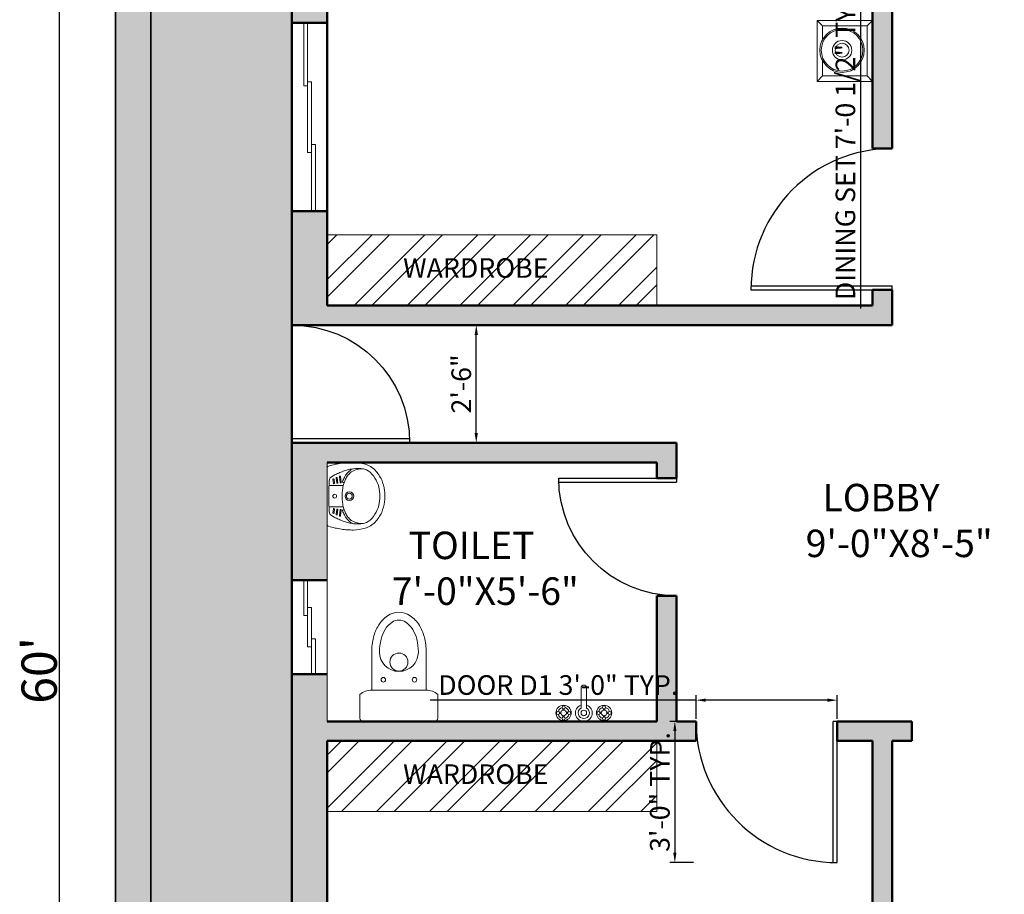
# Model space of a CAD drawing. Units: inches. Extents: x 1734 to 4011, y 1071 to 1891.
# Tile 16 of 27: x 3092 to 3343, y 1415 to 1638. Entities that reach past the tile are written whole.
import ezdxf

# ---------------------------------------------------------------- set-up
doc = ezdxf.new("R2010")
doc.units = ezdxf.units.IN
for name, color, linetype, lineweight in [('0.15', 34, 'Continuous', 15), ('A-ANNO-DIMS', 2, 'Continuous', 18), ('A-AREA-IDEN', 3, 'Continuous', 18), ('A-DOOR', 3, 'Continuous', 25), ('A-FLOR-FIXT', 9, 'Continuous', 18), ('A-FLOR-PATT', 252, 'Continuous', 13), ('A-FURN', 8, 'Continuous', 18), ('A-FURN-PATT', 252, 'Continuous', 13), ('A-GLAZ', 4, 'Continuous', 18), ('A-WALL', 7, 'Continuous', 50), ('A-WALL-PATT', 8, 'Continuous', 13), ('C-PROP', 1, 'Continuous', 35)]:
    doc.layers.add(name, color=color, linetype=linetype, lineweight=lineweight)
doc.styles.get("Standard").update_dxf_attribs({"font": 'arial.ttf'})
doc.dimstyles.new('ISO-25', dxfattribs={"dimtxt": 5, "dimasz": 2.5, "dimexe": 1.25, "dimexo": 0.625, "dimtad": 1, "dimdec": 1, "dimlunit": 3, "dimtxsty": 'Standard', "dimcen": 2.5, "dimclrt": 1, "dimadec": 0, "dimazin": 0, "dimtfac": 1, "dimtdec": 1, "dimtmove": 0, "dimatfit": 3, "dimfxl": 1, "dimarcsym": 0})
pattern_1 = [(45, (1357.344, -12.241), (-6.735192, 6.735192), []), (45, (1361.834, -12.241), (-6.735192, 6.735192), [])]

# ---------------------------------------------------------------- blocks, each defined once
blk = doc.blocks.new('*D58')
at = {"layer": 'A-ANNO-DIMS', "color": 0, "lineweight": -2, "transparency": 16777216}
for p, q in [((3207.88, 1559.82), (3206.72, 1559.82)), ((3207.97, 1532.32), (3207.97, 1557.32)), ((3207.88, 1529.82), (3206.72, 1529.82))]:
    blk.add_line(p, q, dxfattribs=at)
at = {"layer": 'A-ANNO-DIMS', "color": 0, "transparency": 16777216}
for points in [[(3207.55, 1557.32), (3208.39, 1557.32), (3207.97, 1559.82)], [(3207.55, 1532.32), (3208.39, 1532.32), (3207.97, 1529.82)]]:
    blk.add_solid(points, dxfattribs=at)
at = {"layer": 'Defpoints', "color": 0, "transparency": 16777216}
for p in [(3207.97, 1559.82), (3208.51, 1559.82), (3208.51, 1529.82)]:
    blk.add_point(p, dxfattribs=at)
at = {"layer": 'A-ANNO-DIMS', "color": 0, "transparency": 16777216, "insert": (3204.79, 1544.82), "char_height": 5, "attachment_point": 5, "rotation": 90}
blk.add_mtext('2\'-6"', dxfattribs=at)
blk = doc.blocks.new('*D66')
at = {"layer": 'A-ANNO-DIMS', "color": 0, "lineweight": -2, "transparency": 16777216}
for p, q in [((3115.37, 1831.82), (3100.52, 1831.82)), ((3101.77, 1114.32), (3101.77, 1829.32)), ((3115.37, 1111.82), (3100.52, 1111.82))]:
    blk.add_line(p, q, dxfattribs=at)
at = {"layer": 'A-ANNO-DIMS', "color": 0, "transparency": 16777216}
for points in [[(3101.36, 1829.32), (3102.19, 1829.32), (3101.77, 1831.82)], [(3101.36, 1114.32), (3102.19, 1114.32), (3101.77, 1111.82)]]:
    blk.add_solid(points, dxfattribs=at)
at = {"layer": 'Defpoints', "color": 0, "transparency": 16777216}
for p in [(3101.77, 1831.82), (3115.99, 1831.82), (3115.99, 1111.82)]:
    blk.add_point(p, dxfattribs=at)
at = {"layer": 'A-ANNO-DIMS', "color": 0, "transparency": 16777216, "insert": (3096.55, 1471.82), "char_height": 5, "attachment_point": 5, "rotation": 90}
blk.add_mtext("{\\H1.8x;60'}", dxfattribs=at)
blk = doc.blocks.new("D1 3'")
for p, q in [((0, 36), (0, 0)), ((1, 36), (1, 0)), ((0, 0), (1, 0))]:
    blk.add_line(p, q)
blk.add_arc((0, 0), 36, 0, 90)
blk = doc.blocks.new("D2 2'6")
for p, q in [((0, 30), (0, 0)), ((1, 30), (1, 0)), ((0, 0), (1, 0))]:
    blk.add_line(p, q)
blk.add_arc((0, 0), 30, 0, 90)
blk = doc.blocks.new('VELADOR')
at = {"layer": '0.15'}
for p, q in [((-0.2475, 0), (-0.2025, -0.045)), ((0.2475, 0), (0.2025, -0.045)), ((-0.2025, -0.405), (-0.2475, -0.45)), ((0.2475, -0.45), (0.2025, -0.405))]:
    blk.add_line(p, q, dxfattribs=at)
blk.add_lwpolyline([(-0.2475, 0), (-0.2475, -0.45), (0.2475, -0.45), (0.2475, 0)], close=True, dxfattribs=at)
blk.add_lwpolyline([(0.0921, -0.405), (0.2025, -0.405), (0.2025, -0.045), (-0.2025, -0.045), (-0.2025, -0.405), (-0.0818, -0.405)], dxfattribs=at)
for radius in [0.18, 0.1688, 0.0788, 0.0563]:
    blk.add_circle((0.0052, -0.2474), radius, dxfattribs=at)
blk = doc.blocks.new('lavamanos 2')
at = {"layer": '0.15'}
for p, q in [((0, 0.2335), (0, -0.2335)), ((-0.1304, 0.11), (-0.1315, 0.11)), ((-0.0142, 0.087), (-0.13, 0.086)), ((-0.1127, 0.112), (-0.1067, 0.1581)), ((-0.1037, 0.1109), (-0.0978, 0.157)), ((-0.0857, 0.1085), (-0.0807, 0.1466)), ((-0.0767, 0.1074), (-0.0718, 0.1455)), ((-0.0587, 0.105), (-0.0548, 0.1351)), ((-0.0497, 0.1039), (-0.0458, 0.134)), ((-0.1304, -0.11), (-0.1315, -0.11)), ((-0.0142, -0.087), (-0.13, -0.086)), ((-0.1127, -0.112), (-0.1067, -0.1581)), ((-0.1037, -0.1109), (-0.0978, -0.157)), ((-0.0857, -0.1085), (-0.0807, -0.1466)), ((-0.0767, -0.1074), (-0.0718, -0.1455)), ((-0.0587, -0.105), (-0.0548, -0.1351)), ((-0.0497, -0.1039), (-0.0458, -0.134))]:
    blk.add_line(p, q, dxfattribs=at)
for centre, radius in [((-0.178, 0), 0.035), ((-0.178, 0), 0.0235), ((-0.06, 0), 0.015)]:
    blk.add_circle(centre, radius, dxfattribs=at)
for centre, radius, start, end in [((-0.2419, 0.0663), 0.2023, 108.1945, 135.36859), ((-0.2035, -0.0862), 0.3593, 91.20299, 106.42552), ((-0.2208, -0.6855), 0.9585, 86.55138, 89.41308), ((-0.2121, -0.5476), 0.8204, 83.12241, 86.5796), ((5.8279, 30.215), 30.5319, 258.77821, 258.87599), ((-0.1265, -0.0657), 0.3287, 69.06009, 78.82181), ((-0.0202, 0.212), 0.0314, 54.79491, 69.06009), ((-0.1663, 0.0005), 0.3024, 136.57187, 154.32772), ((-0.2422, 0.0655), 0.1638, 121.99295, 150.58892), ((-0.2657, 0.1037), 0.119, 92.47742, 122.14108), ((-0.2765, 0.0677), 0.1528, 57.2491, 95.54005), ((-0.2442, -0.0128), 0.2368, 77.24819, 96.46321), ((-0.2765, 0.0677), 0.1678, 56.87663, 64.99714), ((-0.3662, -0.002), 0.2627, 40.35252, 49.00458), ((-0.2222, 0.0026), 0.2177, 71.98488, 82.01242), ((-0.3662, -0.002), 0.2777, 40.35252, 49.22548), ((-0.2374, 0.11), 0.0921, 27.31862, 39.11562), ((-0.3103, -0.315), 0.5472, 69.51913, 73.49118), ((-0.2374, 0.11), 0.1071, 27.57433, 39.11562), ((-0.3494, 0.0363), 0.2408, 22.19214, 30.78376), ((-0.2991, -0.2855), 0.5156, 65.23004, 69.53785), ((-0.1022, 0.1575), 0.0045, 352.61396, 172.61396), ((-0.2784, -0.2408), 0.4663, 60.24131, 65.2382), ((-0.0648, 0.1184), 0.049, 1.58272, 68.62081), ((-0.005, 0.2335), 0.005, 0, 54.79491), ((-0.0557, -0.0178), 0.4111, 158.70106, 171.31016), ((-0.1999, 0.0263), 0.2202, 147.11565, 167.44248), ((-0.3494, 0.0363), 0.2258, 22.33605, 30.8927), ((-1.2664, -0.2389), 1.1824, 16.36313, 17.77674), ((-0.1315, 0.117), 0.007, 197.40991, 270.49494), ((0.1853, 0.1648), 0.325, 192.53887, 196.70718), ((-0.1305, 0.117), 0.007, 270.49494, 17.39527), ((-1.2664, -0.2389), 1.1974, 17.39527, 17.80495), ((-0.1082, 0.1115), 0.0045, 172.61396, 352.61396), ((-0.0812, 0.108), 0.0045, 172.61396, 352.61396), ((-0.0763, 0.146), 0.0045, 352.61396, 172.61396), ((-0.0542, 0.1045), 0.0045, 172.61396, 352.61396), ((-0.0503, 0.1345), 0.0045, 352.61396, 172.61396), ((-2.1477, 0.0009), 2.1352, 359.97535, 3.19009), ((-0.2093, 0.0056), 0.2558, 171.31016, 181.26266), ((-0.2093, -0.0056), 0.2558, 178.73734, 188.68984), ((0.4664, -0.0834), 0.8953, 169.86317, 174.65802), ((0.4664, 0.0834), 0.8953, 185.34198, 190.13683), ((0.3887, 0.121), 0.517, 185.50529, 189.81306), ((-0.7181, -0.0071), 0.5987, 0.67647, 3.82165), ((-0.7181, 0.0071), 0.5987, 356.17835, 359.32353), ((-2.1477, -0.0009), 2.1352, 356.80991, 0.02465), ((-0.0557, 0.0178), 0.4111, 188.68984, 201.29894), ((-0.1999, -0.0263), 0.2202, 192.55752, 212.88435), ((0.1853, -0.1648), 0.325, 163.29282, 167.46113), ((0.3887, -0.1209), 0.517, 170.18694, 174.49471), ((-0.1663, -0.0005), 0.3024, 205.67228, 223.42813), ((-0.2422, -0.0655), 0.1638, 209.41108, 238.00705), ((-0.2374, -0.1099), 0.0921, 320.88438, 332.68138), ((-0.3494, -0.0363), 0.2258, 329.1073, 337.66395), ((-0.3494, -0.0363), 0.2408, 329.21624, 337.80786), ((-1.2664, 0.2389), 1.1824, 342.22326, 343.63687), ((-0.1315, -0.117), 0.007, 89.50506, 162.59009), ((-0.1305, -0.117), 0.007, 342.60473, 89.50506), ((-1.2664, 0.2389), 1.1974, 342.19505, 342.60473), ((-0.1082, -0.1115), 0.0045, 7.38604, 187.38604), ((-0.1022, -0.1575), 0.0045, 187.38604, 7.38604), ((-0.0812, -0.108), 0.0045, 7.38604, 187.38604), ((-0.0763, -0.146), 0.0045, 187.38604, 7.38604), ((-0.0542, -0.1045), 0.0045, 7.38604, 187.38604), ((-0.0503, -0.1345), 0.0045, 187.38604, 7.38604), ((-0.0648, -0.1184), 0.049, 291.37919, 358.41728), ((-0.2419, -0.0663), 0.2023, 224.63141, 251.8055), ((-0.2657, -0.1036), 0.119, 237.85892, 267.52258), ((-0.2765, -0.0677), 0.1528, 264.45995, 302.7509), ((-0.2442, 0.0128), 0.2368, 263.53679, 282.75181), ((-0.2765, -0.0677), 0.1678, 295.00286, 303.12337), ((-0.3662, 0.002), 0.2627, 310.99542, 319.64748), ((-0.2222, -0.0026), 0.2177, 277.98758, 288.01512), ((-0.3662, 0.002), 0.2777, 310.77452, 319.64748), ((-0.3103, 0.315), 0.5472, 286.50882, 290.48087), ((-0.2374, -0.1099), 0.1071, 320.88438, 332.42567), ((-0.2991, 0.2855), 0.5156, 290.46215, 294.76996), ((-0.2784, 0.2408), 0.4663, 294.7618, 299.75869), ((-0.0202, -0.212), 0.0314, 290.93991, 305.20509), ((-0.005, -0.2335), 0.005, 305.20509, 0), ((-0.2035, 0.0862), 0.3593, 253.57448, 268.79701), ((-0.2208, 0.6855), 0.9585, 270.58692, 273.44862), ((-0.2121, 0.5476), 0.8204, 273.4204, 276.87759), ((5.8279, -30.215), 30.5319, 101.12401, 101.22179), ((-0.1265, 0.0657), 0.3287, 281.17819, 290.93991)]:
    blk.add_arc(centre, radius, start, end, dxfattribs=at)
blk = doc.blocks.new('rreerr')
blk.add_lwpolyline([(2512.8529, 833.5601, 0.205217), (2512.9279, 833.5883), (2512.9279, 833.7401, 0.414214), (2512.9079, 833.7601), (2512.4479, 833.7601, 0.414214), (2512.4279, 833.7401), (2512.4279, 833.5883, 0.205217), (2512.5029, 833.5601)], format="xyb")
for points in [[(2512.5468, 833.1438, 0.107027), (2512.6056, 833.0819, 0.150548), (2512.6779, 833.0596, 0.150548), (2512.7502, 833.0819, 0.107027), (2512.809, 833.1438, 0.075071), (2512.8412, 833.2206, 0.0618), (2512.8529, 833.3151), (2512.8529, 833.5601), (2512.5029, 833.5601), (2512.5029, 833.3151, 0.0618), (2512.5146, 833.2206, 0.075071)], [(2512.5631, 833.2328, 0.075071), (2512.5895, 833.1698, 0.107027), (2512.6338, 833.1232, 0.150548), (2512.6779, 833.1096, 0.150548), (2512.722, 833.1232, 0.107027), (2512.7663, 833.1698, 0.075071), (2512.7927, 833.2328, 0.0618), (2512.8029, 833.3151, 1), (2512.5529, 833.3151, 0.0618)]]:
    blk.add_lwpolyline(points, format="xyb", close=True)
for centre, radius in [((2512.5779, 833.493), 0.0146), ((2512.7779, 833.493), 0.0146), ((2512.6775, 833.3793), 0.0579)]:
    blk.add_circle(centre, radius)
blk = doc.blocks.new('Faucet - Bathroom top')
for p, q in [((-4.107, 0.125), (-4.375, 0.125)), ((-3.75, 0.4788), (-3.75, 0.75)), ((-3.5, 0.482), (-3.5, 0.75)), ((-3.1461, 0.125), (-2.875, 0.125)), ((3.143, 0.125), (2.875, 0.125)), ((3.5, 0.4788), (3.5, 0.75)), ((3.75, 0.482), (3.75, 0.75)), ((4.1039, 0.125), (4.375, 0.125)), ((-4.1039, -0.125), (-4.375, -0.125)), ((-3.75, -0.4821), (-3.75, -0.75)), ((-3.5, -0.4789), (-3.5, -0.75)), ((-3.143, -0.125), (-2.875, -0.125)), ((-0.5, -0.8639), (-0.5, -4.5)), ((0.5, -4.5), (0.5, -0.8631)), ((3.1461, -0.125), (2.875, -0.125)), ((3.5, -0.4821), (3.5, -0.75)), ((3.75, -0.4789), (3.75, -0.75)), ((4.107, -0.125), (4.375, -0.125))]:
    blk.add_line(p, q)
for centre, radius in [((-3.625, 0), 1.375), ((-4.625, 0), 0.2795), ((-3.625, 0), 0.5), ((-3.625, 1), 0.2795), ((-2.625, 0), 0.2795), ((0, 0), 0.5), ((3.625, 0), 1.375), ((2.625, 0), 0.2795), ((3.625, 0), 0.5), ((3.625, 1), 0.2795), ((4.625, 0), 0.2795), ((-3.625, -1), 0.2795), ((3.625, -1), 0.2795)]:
    blk.add_circle(centre, radius)
for centre, radius, start, end in [((-3.625, 0), 1, 105.2407, 164.2093), ((-3.625, 0), 1, 16.44125, 74.07887), ((0, 0), 1.5, 289.6514, 250.3603), ((0, 0), 1, 300.3431, 239.7554), ((3.625, 0), 1, 106.12, 164.0884), ((3.625, 0), 1, 16.23422, 73.90469), ((-3.625, 0), 1, 196.2342, 253.9047), ((-3.625, 0), 1, 286.12, 344.0884), ((3.625, 0), 1, 196.4413, 254.0789), ((3.625, 0), 1, 285.2407, 344.2093), ((0, -4.5), 0.5, 180, 0)]:
    blk.add_arc(centre, radius, start, end)
blk = doc.blocks.new('*D73')
at = {"layer": 'A-ANNO-DIMS', "color": 0, "lineweight": -2, "transparency": 16777216}
for p, q in [((3263.99, 1464.22), (3196.25, 1464.22)), ((3263.99, 1459.44), (3263.99, 1465.47)), ((3297.49, 1464.22), (3266.49, 1464.22)), ((3299.99, 1459.44), (3299.99, 1465.47))]:
    blk.add_line(p, q, dxfattribs=at)
at = {"layer": 'A-ANNO-DIMS', "color": 0, "transparency": 16777216}
for points in [[(3266.49, 1464.64), (3266.49, 1463.8), (3263.99, 1464.22)], [(3297.49, 1464.64), (3297.49, 1463.8), (3299.99, 1464.22)]]:
    blk.add_solid(points, dxfattribs=at)
at = {"layer": 'Defpoints', "color": 0, "transparency": 16777216}
for p in [(3263.99, 1464.22), (3263.99, 1458.82), (3299.99, 1458.82)]:
    blk.add_point(p, dxfattribs=at)
at = {"layer": 'A-ANNO-DIMS', "color": 1, "transparency": 16777216, "insert": (3228.87, 1467.43), "char_height": 5, "attachment_point": 5}
blk.add_mtext('DOOR D1 3\'-0" TYP.', dxfattribs=at)
blk = doc.blocks.new('*D74')
at = {"layer": 'A-ANNO-DIMS', "color": 0, "lineweight": -2, "transparency": 16777216}
for p, q in [((3263.37, 1458.82), (3257.34, 1458.82)), ((3258.59, 1456.32), (3258.59, 1425.32)), ((3263.37, 1422.82), (3257.34, 1422.82))]:
    blk.add_line(p, q, dxfattribs=at)
at = {"layer": 'A-ANNO-DIMS', "color": 0, "transparency": 16777216}
for points in [[(3258.18, 1456.32), (3259.01, 1456.32), (3258.59, 1458.82)], [(3258.18, 1425.32), (3259.01, 1425.32), (3258.59, 1422.82)]]:
    blk.add_solid(points, dxfattribs=at)
at = {"layer": 'Defpoints', "color": 0, "transparency": 16777216}
for p in [(3263.99, 1458.82), (3258.59, 1422.82), (3263.99, 1422.82)]:
    blk.add_point(p, dxfattribs=at)
at = {"layer": 'A-ANNO-DIMS', "color": 1, "transparency": 16777216, "insert": (3255.41, 1440.82), "char_height": 5, "attachment_point": 5, "rotation": 90}
blk.add_mtext('3\'-0" TYP.', dxfattribs=at)
blk = doc.blocks.new('*D99')
at = {"layer": 'A-ANNO-DIMS', "color": 0, "lineweight": -2, "transparency": 16777216}
for p, q in [((3317.99, 1736.23), (3304.67, 1736.23)), ((3305.92, 1733.73), (3305.92, 1654.07)), ((3317.99, 1651.57), (3304.67, 1651.57)), ((3305.92, 1651.57), (3305.92, 1564.03))]:
    blk.add_line(p, q, dxfattribs=at)
at = {"layer": 'A-ANNO-DIMS', "color": 0, "transparency": 16777216}
for points in [[(3305.5, 1733.73), (3306.34, 1733.73), (3305.92, 1736.23)], [(3305.5, 1654.07), (3306.34, 1654.07), (3305.92, 1651.57)]]:
    blk.add_solid(points, dxfattribs=at)
at = {"layer": 'Defpoints', "color": 0, "transparency": 16777216}
for p in [(3318.62, 1736.23), (3305.92, 1651.57), (3318.62, 1651.57)]:
    blk.add_point(p, dxfattribs=at)
at = {"layer": 'A-ANNO-DIMS', "color": 1, "transparency": 16777216, "insert": (3302.71, 1606.55), "char_height": 5, "attachment_point": 5, "rotation": 90}
blk.add_mtext('DINING SET 7\'-0 1/2" TYP.', dxfattribs=at)

msp = doc.modelspace()

# ---------------------------------------------------------------- hatches: boundary and pattern name
at = {"layer": 'A-FLOR-PATT'}
h = msp.add_hatch(color=256, dxfattribs=at)
h.dxf.hatch_style = 1
h.paths.add_polyline_path([(3124.99, 1745.82), (3115.99, 1745.82), (3115.99, 1111.82), (3171.99, 1111.82), (3171.99, 1120.82), (3124.99, 1120.82)])
h = msp.add_hatch(color=256, dxfattribs=at)
h.dxf.hatch_style = 1
h.paths.add_polyline_path([(3160.99, 1745.82), (3124.99, 1745.82), (3124.99, 1312.82), (3160.99, 1312.82), (3160.99, 1529.82)])
at = {"layer": 'A-FURN-PATT'}
h = msp.add_hatch(dxfattribs=at)
h.set_pattern_fill('ANSI32', color=256)
h.set_pattern_definition(pattern_1)
h.paths.add_polyline_path([(3308.99, 1822.82), (3219.99, 1822.82), (3219.99, 1804.82), (3308.99, 1804.82)])
h.paths.add_polyline_path([(3253.99, 1453.82), (3169.99, 1453.82), (3169.99, 1435.82), (3253.99, 1435.82)])
h.paths.add_polyline_path([(3183.49, 1440.04), (3232.95, 1440.04), (3232.95, 1450.34), (3183.49, 1450.34)], flags=24)
h = msp.add_hatch(dxfattribs=at)
h.set_pattern_fill('ANSI32', color=256)
h.set_pattern_definition(pattern_1)
h.paths.add_polyline_path([(3253.99, 1582.82), (3169.99, 1582.82), (3169.99, 1564.82), (3253.99, 1564.82)])
h.paths.add_polyline_path([(3183.49, 1569.04), (3232.95, 1569.04), (3232.95, 1579.34), (3183.49, 1579.34)], flags=24)
at = {"layer": 'A-WALL-PATT'}
h = msp.add_hatch(color=256, dxfattribs=at)
h.dxf.hatch_style = 1
h.paths.add_polyline_path([(3475.99, 1831.82), (3115.99, 1831.82), (3115.99, 1745.82), (3130.99, 1745.82), (3130.99, 1750.82), (3124.99, 1750.82), (3124.99, 1822.82), (3214.99, 1822.82), (3214.99, 1780.82), (3219.99, 1780.82), (3219.99, 1822.82), (3308.99, 1822.82), (3308.99, 1750.82), (3254.99, 1750.82), (3254.99, 1745.82), (3308.99, 1745.82), (3308.99, 1604.82), (3313.99, 1604.82), (3313.99, 1745.82), (3366.99, 1745.82), (3366.99, 1750.82), (3313.99, 1750.82), (3313.99, 1822.82), (3401.99, 1822.82), (3401.99, 1750.82), (3396.99, 1750.82), (3396.99, 1745.82), (3411.99, 1745.82), (3411.99, 1750.82), (3406.99, 1750.82), (3406.99, 1822.82), (3466.99, 1822.82), (3466.99, 1750.82), (3441.99, 1750.82), (3441.99, 1745.82), (3466.99, 1745.82), (3466.99, 1517.82), (3452.49, 1517.82), (3452.49, 1512.82), (3466.99, 1512.82), (3466.99, 1458.82), (3446.49, 1458.82), (3446.49, 1453.82), (3466.99, 1453.82), (3466.99, 1237.82), (3372.99, 1237.82), (3372.99, 1228.82), (3466.99, 1228.82), (3466.99, 1120.82), (3309.99, 1120.82), (3309.99, 1184.82), (3310.99, 1184.82), (3310.99, 1189.82), (3303.99, 1189.82), (3303.99, 1120.82), (3291.99, 1120.82), (3291.99, 1111.82), (3475.99, 1111.82)])
h.paths.add_polyline_path([(3169.99, 1745.82), (3224.99, 1745.82), (3224.99, 1750.82), (3154.99, 1750.82), (3154.99, 1745.82), (3160.99, 1745.82), (3160.99, 1636.82), (3169.99, 1636.82)], flags=17)
h.paths.add_polyline_path([(3169.99, 1588.82), (3160.99, 1588.82), (3160.99, 1559.82), (3313.99, 1559.82), (3313.99, 1568.82), (3308.99, 1568.82), (3308.99, 1564.82), (3169.99, 1564.82)], flags=17)
h.paths.add_polyline_path([(3416.49, 1517.82), (3401.99, 1517.82), (3401.99, 1512.82), (3416.49, 1512.82)], flags=17)
h.paths.add_polyline_path([(3371.99, 1517.82), (3366.99, 1517.82), (3366.99, 1453.82), (3392.49, 1453.82), (3392.49, 1458.82), (3371.99, 1458.82)], flags=17)
h.paths.add_polyline_path([(3258.99, 1529.82), (3160.99, 1529.82), (3160.99, 1494.82), (3169.99, 1494.82), (3169.99, 1524.82), (3253.99, 1524.82), (3253.99, 1520.82), (3258.99, 1520.82)], flags=17)
h.paths.add_polyline_path([(3263.99, 1458.82), (3258.99, 1458.82), (3258.99, 1490.82), (3253.99, 1490.82), (3253.99, 1458.82), (3169.99, 1458.82), (3169.99, 1470.82), (3160.99, 1470.82), (3160.99, 1387.82), (3169.99, 1387.82), (3169.99, 1453.82), (3263.99, 1453.82)], flags=17)
h.paths.add_polyline_path([(3313.99, 1453.82), (3318.99, 1453.82), (3318.99, 1458.82), (3299.99, 1458.82), (3299.99, 1453.82), (3308.99, 1453.82), (3308.99, 1321.82), (3266.49, 1321.82), (3266.49, 1312.82), (3313.99, 1312.82)], flags=17)
h.paths.add_polyline_path([(3212.49, 1321.82), (3169.99, 1321.82), (3169.99, 1339.82), (3160.99, 1339.82), (3160.99, 1312.82), (3212.49, 1312.82)], flags=17)
h.paths.add_polyline_path([(3313.99, 1288.82), (3304.99, 1288.82), (3304.99, 1285.82), (3313.99, 1285.82)], flags=17)
h.paths.add_polyline_path([(3324.99, 1237.82), (3304.99, 1237.82), (3304.99, 1228.82), (3324.99, 1228.82)], flags=17)

# ---------------------------------------------------------------- linework, layer by layer
at = {"layer": 'A-FURN'}
for p, q in [((3169.99, 1582.82), (3253.99, 1582.82)), ((3253.99, 1564.82), (3253.99, 1582.82)), ((3169.99, 1458.82), (3169.99, 1524.82)), ((3169.99, 1435.82), (3253.99, 1435.82))]:
    msp.add_line(p, q, dxfattribs=at)
at = {"layer": 'A-GLAZ'}
for p, q in [((3163.99, 1636.82), (3163.99, 1620.82)), ((3164.99, 1636.82), (3164.99, 1603.82)), ((3164.99, 1621.82), (3165.99, 1621.82)), ((3165.99, 1621.82), (3165.99, 1588.82)), ((3163.99, 1620.82), (3164.99, 1620.82)), ((3165.99, 1605.82), (3166.99, 1605.82)), ((3166.99, 1605.82), (3166.99, 1588.82)), ((3164.99, 1603.82), (3165.99, 1603.82)), ((3163.99, 1485.82), (3163.99, 1494.82)), ((3164.99, 1477.82), (3164.99, 1494.82)), ((3165.99, 1487.82), (3164.99, 1487.82)), ((3165.99, 1470.82), (3165.99, 1487.82)), ((3164.99, 1485.82), (3163.99, 1485.82)), ((3166.99, 1479.82), (3165.99, 1479.82)), ((3166.99, 1470.82), (3166.99, 1479.82)), ((3165.99, 1477.82), (3164.99, 1477.82)), ((3253.99, 1435.82), (3253.99, 1453.82))]:
    msp.add_line(p, q, dxfattribs=at)
at = {"layer": 'A-WALL'}
for p, q in [((3160.99, 1529.82), (3160.99, 1745.82)), ((3169.99, 1564.82), (3169.99, 1745.82)), ((3308.99, 1604.82), (3308.99, 1745.82)), ((3313.99, 1604.82), (3313.99, 1745.82)), ((3160.99, 1636.82), (3169.99, 1636.82)), ((3308.99, 1604.82), (3313.99, 1604.82)), ((3160.99, 1588.82), (3169.99, 1588.82)), ((3308.99, 1568.82), (3313.99, 1568.82)), ((3308.99, 1564.82), (3308.99, 1568.82)), ((3313.99, 1559.82), (3313.99, 1568.82)), ((3169.99, 1564.82), (3308.99, 1564.82)), ((3169.99, 1564.82), (3253.99, 1564.82)), ((3160.99, 1559.82), (3313.99, 1559.82)), ((3160.99, 1529.82), (3258.99, 1529.82)), ((3160.99, 1312.82), (3160.99, 1529.82)), ((3258.99, 1520.82), (3258.99, 1529.82)), ((3169.99, 1524.82), (3253.99, 1524.82)), ((3253.99, 1520.82), (3253.99, 1524.82)), ((3253.99, 1520.82), (3258.99, 1520.82)), ((3169.99, 1494.82), (3160.99, 1494.82)), ((3253.99, 1490.82), (3258.99, 1490.82)), ((3253.99, 1458.82), (3253.99, 1490.82)), ((3258.99, 1458.82), (3258.99, 1490.82)), ((3169.99, 1470.82), (3160.99, 1470.82)), ((3169.99, 1458.82), (3253.99, 1458.82)), ((3258.99, 1458.82), (3263.99, 1458.82)), ((3263.99, 1453.82), (3263.99, 1458.82)), ((3299.99, 1458.82), (3318.99, 1458.82)), ((3299.99, 1453.82), (3299.99, 1458.82)), ((3318.99, 1453.82), (3318.99, 1458.82)), ((3169.99, 1453.82), (3263.99, 1453.82)), ((3169.99, 1321.82), (3169.99, 1453.82)), ((3299.99, 1453.82), (3308.99, 1453.82)), ((3308.99, 1321.82), (3308.99, 1453.82)), ((3313.99, 1453.82), (3318.99, 1453.82)), ((3313.99, 1285.82), (3313.99, 1453.82))]:
    msp.add_line(p, q, dxfattribs=at)
at = {"layer": 'C-PROP'}
msp.add_line((3124.99, 1120.82), (3124.99, 1745.82), dxfattribs=at)
msp.add_lwpolyline([(3171.99, 1111.82), (3115.99, 1111.82), (3115.99, 1831.82), (3475.99, 1831.82), (3475.99, 1111.82), (3291.99, 1111.82)], dxfattribs=at)

# ---------------------------------------------------------------- block references
at = {"layer": 'A-DOOR'}
for p, rotation in [((3313.99, 1568.82), 90), ((3299.99, 1458.82), 180)]:
    msp.add_blockref("D1 3'", p, dxfattribs=dict(at, rotation=rotation))
at = {"layer": 'A-DOOR', "xscale": -1}
for p, rotation in [((3160.99, 1529.82), 270), ((3258.99, 1520.82), 90)]:
    msp.add_blockref("D2 2'6", p, dxfattribs=dict(at, rotation=rotation))
at = {"layer": 'A-FLOR-FIXT'}
for name, p, xscale, yscale, zscale, rotation in [('lavamanos 2', (3169.99, 1516.21), 31.61240364394164, 31.61240364394164, 31.61240364394164, 179.99990349049), ('rreerr', (-96567.57, 34559.93), -39.701, 39.701, 39.701, 180), ('Faucet - Bathroom top', (3235.39, 1460.96), -1.424049708253414, 1.424049708253414, 1.424049708253414, 180)]:
    msp.add_blockref(name, p, dxfattribs=dict(at, xscale=xscale, yscale=yscale, zscale=zscale, rotation=rotation))
at = {"layer": 'A-FURN', "xscale": -31.41542173157097, "yscale": 31.41542173157097, "zscale": 31.41542173157097, "rotation": 269.9999999999999}
msp.add_blockref('VELADOR', (3308.99, 1629.7), dxfattribs=at)

# ---------------------------------------------------------------- texts
at = {"layer": 'A-AREA-IDEN', "attachment_point": 1}
for s, insert, char_height in [('   WARDROBE', (3184.74, 1576.86), 5), ('  LOBBY\\P9\'-0"X8\'-5"', (3291.94, 1519.35), 7), ('  TOILET\\P7\'-0"X5\'-6"', (3186.44, 1507.17), 7), ('   WARDROBE', (3184.74, 1447.86), 5)]:
    msp.add_mtext_dynamic_manual_height_columns(s, width=86.9528, gutter_width=12.5, heights=[0], dxfattribs=dict(at, insert=insert, char_height=char_height))

# ---------------------------------------------------------------- dimensions: what is measured, and where the dimension line sits
at = {"layer": 'A-ANNO-DIMS'}
for base, p1, p2, angle, text, override, picture, middle in [((3101.77, 1831.82), (3115.99, 1111.82), (3115.99, 1831.82), 90, '{\\H1.8x;<>}', {"dimclrd": 0, "dimclre": 0, "dimclrt": 0}, '*D66', (3096.55, 1471.82)), ((3305.92, 1651.57), (3318.62, 1736.23), (3318.62, 1651.57), 270, 'DINING SET <> TYP.', {"dimdec": 1, "dimrnd": 0, "dimzin": 1, "dimlunit": 4, "dimfrac": 2}, '*D99', (3302.71, 1606.55)), ((3263.99, 1464.22), (3299.99, 1458.82), (3263.99, 1458.82), 180, 'DOOR D1 <> TYP.', {"dimdec": 1, "dimrnd": 0, "dimzin": 1, "dimlunit": 4, "dimfrac": 2}, '*D73', (3228.87, 1467.43)), ((3258.59, 1422.82), (3263.99, 1458.82), (3263.99, 1422.82), 270, '<> TYP.', {"dimdec": 1, "dimrnd": 0, "dimzin": 1, "dimlunit": 4, "dimfrac": 2}, '*D74', (3255.41, 1440.82))]:
    dim = msp.add_linear_dim(base=base, p1=p1, p2=p2, angle=angle, text=text, dimstyle='ISO-25', override=override, dxfattribs=at)
    dim.commit()
    dim.dimension.update_dxf_attribs({"geometry": picture, "text_midpoint": middle})
dim = msp.add_linear_dim(base=(3207.97, 1559.82), p1=(3208.51, 1529.82), p2=(3208.51, 1559.82), angle=90, dimstyle='ISO-25', override={"dimclrd": 0, "dimclre": 0, "dimclrt": 0}, dxfattribs=at)
dim.commit()
dim.dimension.update_dxf_attribs({"geometry": '*D58', "text_midpoint": (3204.79, 1544.82)})

doc.saveas('drawing.dxf')
